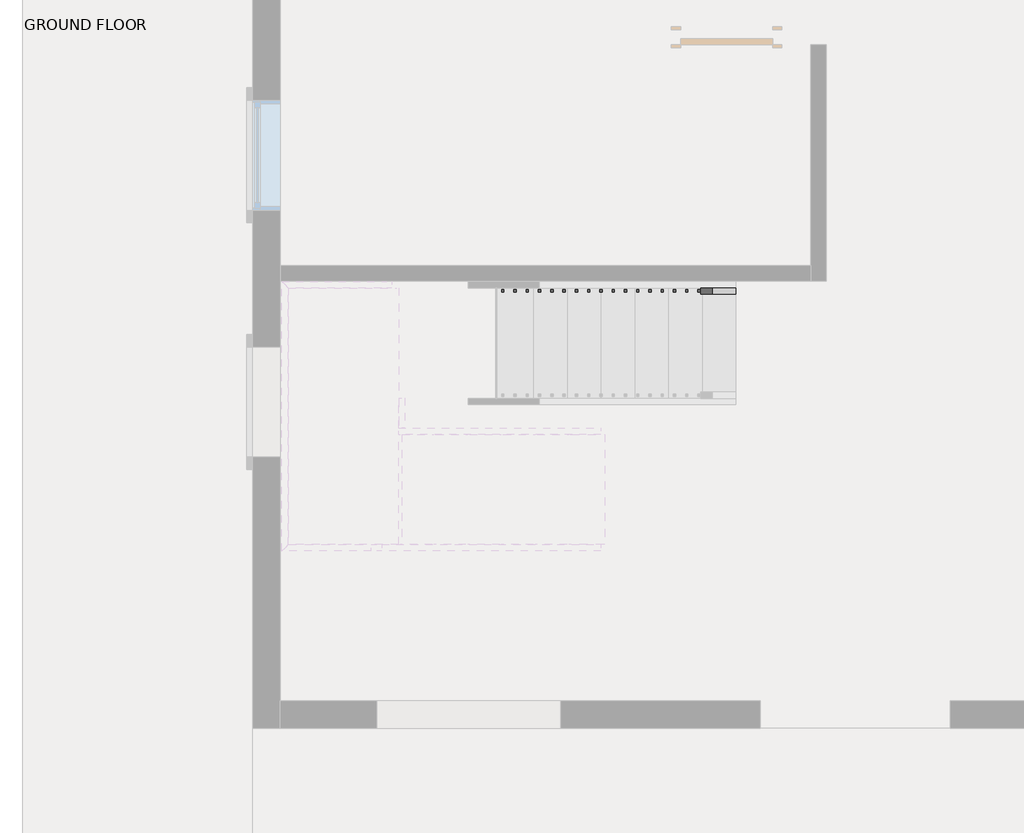
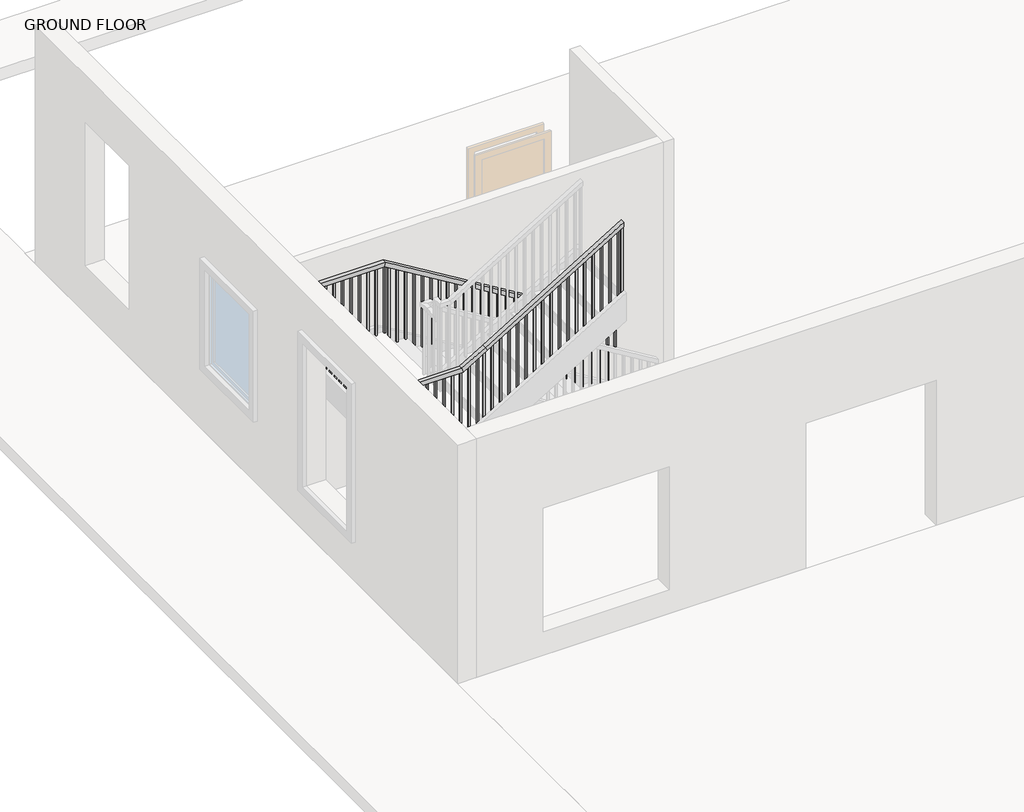
# One storey, part 2 of 3: 1 railing.
"""IFC4 building model written with IfcOpenShell, lengths in millimetres."""

from ifc_helpers import new_model, si_unit, frame, origin, place, context, project, spatial, polyline, outline, extrude, faceted_brep, element, save

model = new_model("IFC4")

# Units and contexts
model_context = context("Model", 3, world=origin())
ifc_project = project(units=[si_unit("LENGTHUNIT", "METRE", prefix="MILLI")], contexts=[model_context])

# Site, building, storey
site = spatial("IfcSite", under=ifc_project)
building = spatial("IfcBuilding", under=site)
storey = spatial("IfcBuildingStorey", under=building, Name="GROUND FLOOR", Elevation=304.8)

# Railing
placement = place(None, origin())
element("IfcRailing", 1, ObjectType="Handrail - Rectangular", at=placement, inside=storey, context=model_context, shape_type="SolidModel", body=[
    faceted_brep([(-5990.8517085, 2868.2826226, 1388.5333333), (-5990.8517085, 2868.2826226, 1329.1318731), (-5990.8517085, 2919.0826226, 1329.1318731), (-5990.8517085, 2919.0826226, 1388.5333333), (-8784.8517085, 2868.2826226, 3081.8666667), (-8799.0441179, 2868.2826226, 3031.0666667), (-8799.0441179, 2919.0826226, 3031.0666667), (-8784.8517085, 2919.0826226, 3081.8666667), (-9648.4517085, 2868.2826226, 3081.8666667), (-9648.4517085, 2868.2826226, 3031.0666667), (-9699.2517085, 2919.0826226, 3031.0666667), (-9699.2517085, 2919.0826226, 3081.8666667), (-9648.4517085, 842.8165128, 3081.8666667), (-9648.4517085, 842.8165128, 3031.0666667), (-9699.2517085, 792.0165128, 3031.0666667), (-9699.2517085, 792.0165128, 3081.8666667), (-9064.2517085, 842.8165128, 3081.8666667), (-9050.0592991, 842.8165128, 3031.0666667), (-9050.0592991, 792.0165128, 3031.0666667), (-9064.2517085, 792.0165128, 3081.8666667), (-8784.8517085, 842.8165128, 3251.2), (-8758.5219813, 842.8165128, 3207.7559502), (-8758.5219813, 792.0165128, 3207.7559502), (-8784.8517085, 792.0165128, 3251.2), (-7108.4517085, 842.8165128, 4267.2), (-7108.4517085, 792.0165128, 4267.2), (-7108.4517085, 792.0165128, 4207.7985397), (-7108.4517085, 842.8165128, 4207.7985397)], [[[0, 1, 2, 3]], [[1, 0, 4, 5]], [[2, 1, 5, 6]], [[3, 2, 6, 7]], [[0, 3, 7, 4]], [[5, 4, 8, 9]], [[6, 5, 9, 10]], [[7, 6, 10, 11]], [[4, 7, 11, 8]], [[9, 8, 12, 13]], [[10, 9, 13, 14]], [[11, 10, 14, 15]], [[8, 11, 15, 12]], [[13, 12, 16, 17]], [[14, 13, 17, 18]], [[15, 14, 18, 19]], [[12, 15, 19, 16]], [[17, 16, 20, 21]], [[18, 17, 21, 22]], [[19, 18, 22, 23]], [[16, 19, 23, 20]], [[24, 25, 26, 27]], [[21, 20, 24, 27]], [[22, 21, 27, 26]], [[23, 22, 26, 25]], [[20, 23, 25, 24]]]),
    extrude(outline(polyline([(4182.7833882, -7149.7267085), (4171.2379337, -7168.7767085), (3183.4666667, -7168.7767085), (3183.4666667, -7149.7267085), (4182.7833882, -7149.7267085)])), frame((0.0, 807.8915128, 0.0), z_axis=(0.0, 1.0, 0.0), x_axis=(0.0, 0.0, 1.0)), (0.0, 0.0, 1.0), 19.05),
    extrude(outline(polyline([(4121.2076307, -7251.3267085), (4109.6621761, -7270.3767085), (3183.4666667, -7270.3767085), (3183.4666667, -7251.3267085), (4121.2076307, -7251.3267085)])), frame((0.0, 807.8915128, 0.0), z_axis=(0.0, 1.0, 0.0), x_axis=(0.0, 0.0, 1.0)), (0.0, 0.0, 1.0), 19.05),
    extrude(outline(polyline([(4059.6318731, -7352.9267085), (4048.0864185, -7371.9767085), (3183.4666667, -7371.9767085), (3183.4666667, -7352.9267085), (4059.6318731, -7352.9267085)])), frame((0.0, 807.8915128, 0.0), z_axis=(0.0, 1.0, 0.0), x_axis=(0.0, 0.0, 1.0)), (0.0, 0.0, 1.0), 19.05),
    extrude(outline(polyline([(3998.0561155, -7454.5267085), (3986.510661, -7473.5767085), (3014.1333333, -7473.5767085), (3014.1333333, -7454.5267085), (3998.0561155, -7454.5267085)])), frame((0.0, 807.8915128, 0.0), z_axis=(0.0, 1.0, 0.0), x_axis=(0.0, 0.0, 1.0)), (0.0, 0.0, 1.0), 19.05),
    extrude(outline(polyline([(3936.4803579, -7556.1267085), (3924.9349034, -7575.1767085), (3014.1333333, -7575.1767085), (3014.1333333, -7556.1267085), (3936.4803579, -7556.1267085)])), frame((0.0, 807.8915128, 0.0), z_axis=(0.0, 1.0, 0.0), x_axis=(0.0, 0.0, 1.0)), (0.0, 0.0, 1.0), 19.05),
    extrude(outline(polyline([(3874.9046004, -7657.7267085), (3863.3591458, -7676.7767085), (3014.1333333, -7676.7767085), (3014.1333333, -7657.7267085), (3874.9046004, -7657.7267085)])), frame((0.0, 807.8915128, 0.0), z_axis=(0.0, 1.0, 0.0), x_axis=(0.0, 0.0, 1.0)), (0.0, 0.0, 1.0), 19.05),
    extrude(outline(polyline([(3813.3288428, -7759.3267085), (3801.7833882, -7778.3767085), (2844.8, -7778.3767085), (2844.8, -7759.3267085), (3813.3288428, -7759.3267085)])), frame((0.0, 807.8915128, 0.0), z_axis=(0.0, 1.0, 0.0), x_axis=(0.0, 0.0, 1.0)), (0.0, 0.0, 1.0), 19.05),
    extrude(outline(polyline([(3751.7530852, -7860.9267085), (3740.2076307, -7879.9767085), (2844.8, -7879.9767085), (2844.8, -7860.9267085), (3751.7530852, -7860.9267085)])), frame((0.0, 807.8915128, 0.0), z_axis=(0.0, 1.0, 0.0), x_axis=(0.0, 0.0, 1.0)), (0.0, 0.0, 1.0), 19.05),
    extrude(outline(polyline([(3690.1773276, -7962.5267085), (3678.6318731, -7981.5767085), (2675.4666667, -7981.5767085), (2675.4666667, -7962.5267085), (3690.1773276, -7962.5267085)])), frame((0.0, 807.8915128, 0.0), z_axis=(0.0, 1.0, 0.0), x_axis=(0.0, 0.0, 1.0)), (0.0, 0.0, 1.0), 19.05),
    extrude(outline(polyline([(3628.60157, -8064.1267085), (3617.0561155, -8083.1767085), (2675.4666667, -8083.1767085), (2675.4666667, -8064.1267085), (3628.60157, -8064.1267085)])), frame((0.0, 807.8915128, 0.0), z_axis=(0.0, 1.0, 0.0), x_axis=(0.0, 0.0, 1.0)), (0.0, 0.0, 1.0), 19.05),
    extrude(outline(polyline([(3567.0258125, -8165.7267085), (3555.4803579, -8184.7767085), (2675.4666667, -8184.7767085), (2675.4666667, -8165.7267085), (3567.0258125, -8165.7267085)])), frame((0.0, 807.8915128, 0.0), z_axis=(0.0, 1.0, 0.0), x_axis=(0.0, 0.0, 1.0)), (0.0, 0.0, 1.0), 19.05),
    extrude(outline(polyline([(3505.4500549, -8267.3267085), (3493.9046004, -8286.3767085), (2506.1333333, -8286.3767085), (2506.1333333, -8267.3267085), (3505.4500549, -8267.3267085)])), frame((0.0, 807.8915128, 0.0), z_axis=(0.0, 1.0, 0.0), x_axis=(0.0, 0.0, 1.0)), (0.0, 0.0, 1.0), 19.05),
    extrude(outline(polyline([(3443.8742973, -8368.9267085), (3432.3288428, -8387.9767085), (2506.1333333, -8387.9767085), (2506.1333333, -8368.9267085), (3443.8742973, -8368.9267085)])), frame((0.0, 807.8915128, 0.0), z_axis=(0.0, 1.0, 0.0), x_axis=(0.0, 0.0, 1.0)), (0.0, 0.0, 1.0), 19.05),
    extrude(outline(polyline([(3382.2985397, -8470.5267085), (3370.7530852, -8489.5767085), (2506.1333333, -8489.5767085), (2506.1333333, -8470.5267085), (3382.2985397, -8470.5267085)])), frame((0.0, 807.8915128, 0.0), z_axis=(0.0, 1.0, 0.0), x_axis=(0.0, 0.0, 1.0)), (0.0, 0.0, 1.0), 19.05),
    extrude(outline(polyline([(3320.7227822, -8572.1267085), (3309.1773276, -8591.1767085), (2336.8, -8591.1767085), (2336.8, -8572.1267085), (3320.7227822, -8572.1267085)])), frame((0.0, 807.8915128, 0.0), z_axis=(0.0, 1.0, 0.0), x_axis=(0.0, 0.0, 1.0)), (0.0, 0.0, 1.0), 19.05),
    extrude(outline(polyline([(3259.1470246, -8673.7267085), (3247.60157, -8692.7767085), (2336.8, -8692.7767085), (2336.8, -8673.7267085), (3259.1470246, -8673.7267085)])), frame((0.0, 807.8915128, 0.0), z_axis=(0.0, 1.0, 0.0), x_axis=(0.0, 0.0, 1.0)), (0.0, 0.0, 1.0), 19.05),
    extrude(outline(polyline([(3151.3894488, -8851.5267085), (3139.8439943, -8870.5767085), (2167.4666667, -8870.5767085), (2167.4666667, -8851.5267085), (3151.3894488, -8851.5267085)])), frame((0.0, 807.8915128, 0.0), z_axis=(0.0, 1.0, 0.0), x_axis=(0.0, 0.0, 1.0)), (0.0, 0.0, 1.0), 19.05),
    extrude(outline(polyline([(3089.8136913, -8953.1267085), (3078.2682367, -8972.1767085), (2167.4666667, -8972.1767085), (2167.4666667, -8953.1267085), (3089.8136913, -8953.1267085)])), frame((0.0, 807.8915128, 0.0), z_axis=(0.0, 1.0, 0.0), x_axis=(0.0, 0.0, 1.0)), (0.0, 0.0, 1.0), 19.05),
    extrude(outline(polyline([(-9073.7767085, 807.8915128), (-9073.7767085, 826.9415128), (-9054.7267085, 826.9415128), (-9054.7267085, 807.8915128), (-9073.7767085, 807.8915128)])), frame((0.0, 0.0, 2167.4666667), z_axis=(0.0, 0.0, 1.0), x_axis=(1.0, 0.0, 0.0)), (0.0, 0.0, 1.0), 863.6),
    extrude(outline(polyline([(-9175.3767085, 807.8915128), (-9175.3767085, 826.9415128), (-9156.3267085, 826.9415128), (-9156.3267085, 807.8915128), (-9175.3767085, 807.8915128)])), frame((0.0, 0.0, 2167.4666667), z_axis=(0.0, 0.0, 1.0), x_axis=(1.0, 0.0, 0.0)), (0.0, 0.0, 1.0), 863.6),
    extrude(outline(polyline([(-9276.9767085, 807.8915128), (-9276.9767085, 826.9415128), (-9257.9267085, 826.9415128), (-9257.9267085, 807.8915128), (-9276.9767085, 807.8915128)])), frame((0.0, 0.0, 2167.4666667), z_axis=(0.0, 0.0, 1.0), x_axis=(1.0, 0.0, 0.0)), (0.0, 0.0, 1.0), 863.6),
    extrude(outline(polyline([(-9378.5767085, 807.8915128), (-9378.5767085, 826.9415128), (-9359.5267085, 826.9415128), (-9359.5267085, 807.8915128), (-9378.5767085, 807.8915128)])), frame((0.0, 0.0, 2167.4666667), z_axis=(0.0, 0.0, 1.0), x_axis=(1.0, 0.0, 0.0)), (0.0, 0.0, 1.0), 863.6),
    extrude(outline(polyline([(-9480.1767085, 807.8915128), (-9480.1767085, 826.9415128), (-9461.1267085, 826.9415128), (-9461.1267085, 807.8915128), (-9480.1767085, 807.8915128)])), frame((0.0, 0.0, 2167.4666667), z_axis=(0.0, 0.0, 1.0), x_axis=(1.0, 0.0, 0.0)), (0.0, 0.0, 1.0), 863.6),
    extrude(outline(polyline([(-9581.7767085, 807.8915128), (-9581.7767085, 826.9415128), (-9562.7267085, 826.9415128), (-9562.7267085, 807.8915128), (-9581.7767085, 807.8915128)])), frame((0.0, 0.0, 2167.4666667), z_axis=(0.0, 0.0, 1.0), x_axis=(1.0, 0.0, 0.0)), (0.0, 0.0, 1.0), 863.6),
    extrude(outline(polyline([(-9683.3767085, 871.2076226), (-9664.3267085, 871.2076226), (-9664.3267085, 852.1576226), (-9683.3767085, 852.1576226), (-9683.3767085, 871.2076226)])), frame((0.0, 0.0, 2167.4666667), z_axis=(0.0, 0.0, 1.0), x_axis=(1.0, 0.0, 0.0)), (0.0, 0.0, 1.0), 863.6),
    extrude(outline(polyline([(-9683.3767085, 972.8076226), (-9664.3267085, 972.8076226), (-9664.3267085, 953.7576226), (-9683.3767085, 953.7576226), (-9683.3767085, 972.8076226)])), frame((0.0, 0.0, 2167.4666667), z_axis=(0.0, 0.0, 1.0), x_axis=(1.0, 0.0, 0.0)), (0.0, 0.0, 1.0), 863.6),
    extrude(outline(polyline([(-9683.3767085, 1074.4076226), (-9664.3267085, 1074.4076226), (-9664.3267085, 1055.3576226), (-9683.3767085, 1055.3576226), (-9683.3767085, 1074.4076226)])), frame((0.0, 0.0, 2167.4666667), z_axis=(0.0, 0.0, 1.0), x_axis=(1.0, 0.0, 0.0)), (0.0, 0.0, 1.0), 863.6),
    extrude(outline(polyline([(-9683.3767085, 1176.0076226), (-9664.3267085, 1176.0076226), (-9664.3267085, 1156.9576226), (-9683.3767085, 1156.9576226), (-9683.3767085, 1176.0076226)])), frame((0.0, 0.0, 2167.4666667), z_axis=(0.0, 0.0, 1.0), x_axis=(1.0, 0.0, 0.0)), (0.0, 0.0, 1.0), 863.6),
    extrude(outline(polyline([(-9683.3767085, 1277.6076226), (-9664.3267085, 1277.6076226), (-9664.3267085, 1258.5576226), (-9683.3767085, 1258.5576226), (-9683.3767085, 1277.6076226)])), frame((0.0, 0.0, 2167.4666667), z_axis=(0.0, 0.0, 1.0), x_axis=(1.0, 0.0, 0.0)), (0.0, 0.0, 1.0), 863.6),
    extrude(outline(polyline([(-9683.3767085, 1379.2076226), (-9664.3267085, 1379.2076226), (-9664.3267085, 1360.1576226), (-9683.3767085, 1360.1576226), (-9683.3767085, 1379.2076226)])), frame((0.0, 0.0, 2167.4666667), z_axis=(0.0, 0.0, 1.0), x_axis=(1.0, 0.0, 0.0)), (0.0, 0.0, 1.0), 863.6),
    extrude(outline(polyline([(-9683.3767085, 1480.8076226), (-9664.3267085, 1480.8076226), (-9664.3267085, 1461.7576226), (-9683.3767085, 1461.7576226), (-9683.3767085, 1480.8076226)])), frame((0.0, 0.0, 2167.4666667), z_axis=(0.0, 0.0, 1.0), x_axis=(1.0, 0.0, 0.0)), (0.0, 0.0, 1.0), 863.6),
    extrude(outline(polyline([(-9683.3767085, 1582.4076226), (-9664.3267085, 1582.4076226), (-9664.3267085, 1563.3576226), (-9683.3767085, 1563.3576226), (-9683.3767085, 1582.4076226)])), frame((0.0, 0.0, 2167.4666667), z_axis=(0.0, 0.0, 1.0), x_axis=(1.0, 0.0, 0.0)), (0.0, 0.0, 1.0), 863.6),
    extrude(outline(polyline([(-9683.3767085, 1684.0076226), (-9664.3267085, 1684.0076226), (-9664.3267085, 1664.9576226), (-9683.3767085, 1664.9576226), (-9683.3767085, 1684.0076226)])), frame((0.0, 0.0, 2167.4666667), z_axis=(0.0, 0.0, 1.0), x_axis=(1.0, 0.0, 0.0)), (0.0, 0.0, 1.0), 863.6),
    extrude(outline(polyline([(-9683.3767085, 1785.6076226), (-9664.3267085, 1785.6076226), (-9664.3267085, 1766.5576226), (-9683.3767085, 1766.5576226), (-9683.3767085, 1785.6076226)])), frame((0.0, 0.0, 2167.4666667), z_axis=(0.0, 0.0, 1.0), x_axis=(1.0, 0.0, 0.0)), (0.0, 0.0, 1.0), 863.6),
    extrude(outline(polyline([(-9683.3767085, 1887.2076226), (-9664.3267085, 1887.2076226), (-9664.3267085, 1868.1576226), (-9683.3767085, 1868.1576226), (-9683.3767085, 1887.2076226)])), frame((0.0, 0.0, 2167.4666667), z_axis=(0.0, 0.0, 1.0), x_axis=(1.0, 0.0, 0.0)), (0.0, 0.0, 1.0), 863.6),
    extrude(outline(polyline([(-9683.3767085, 1988.8076226), (-9664.3267085, 1988.8076226), (-9664.3267085, 1969.7576226), (-9683.3767085, 1969.7576226), (-9683.3767085, 1988.8076226)])), frame((0.0, 0.0, 2167.4666667), z_axis=(0.0, 0.0, 1.0), x_axis=(1.0, 0.0, 0.0)), (0.0, 0.0, 1.0), 863.6),
    extrude(outline(polyline([(-9683.3767085, 2090.4076226), (-9664.3267085, 2090.4076226), (-9664.3267085, 2071.3576226), (-9683.3767085, 2071.3576226), (-9683.3767085, 2090.4076226)])), frame((0.0, 0.0, 2167.4666667), z_axis=(0.0, 0.0, 1.0), x_axis=(1.0, 0.0, 0.0)), (0.0, 0.0, 1.0), 863.6),
    extrude(outline(polyline([(-9683.3767085, 2192.0076226), (-9664.3267085, 2192.0076226), (-9664.3267085, 2172.9576226), (-9683.3767085, 2172.9576226), (-9683.3767085, 2192.0076226)])), frame((0.0, 0.0, 2167.4666667), z_axis=(0.0, 0.0, 1.0), x_axis=(1.0, 0.0, 0.0)), (0.0, 0.0, 1.0), 863.6),
    extrude(outline(polyline([(-9683.3767085, 2293.6076226), (-9664.3267085, 2293.6076226), (-9664.3267085, 2274.5576226), (-9683.3767085, 2274.5576226), (-9683.3767085, 2293.6076226)])), frame((0.0, 0.0, 2167.4666667), z_axis=(0.0, 0.0, 1.0), x_axis=(1.0, 0.0, 0.0)), (0.0, 0.0, 1.0), 863.6),
    extrude(outline(polyline([(-9683.3767085, 2395.2076226), (-9664.3267085, 2395.2076226), (-9664.3267085, 2376.1576226), (-9683.3767085, 2376.1576226), (-9683.3767085, 2395.2076226)])), frame((0.0, 0.0, 2167.4666667), z_axis=(0.0, 0.0, 1.0), x_axis=(1.0, 0.0, 0.0)), (0.0, 0.0, 1.0), 863.6),
    extrude(outline(polyline([(-9683.3767085, 2496.8076226), (-9664.3267085, 2496.8076226), (-9664.3267085, 2477.7576226), (-9683.3767085, 2477.7576226), (-9683.3767085, 2496.8076226)])), frame((0.0, 0.0, 2167.4666667), z_axis=(0.0, 0.0, 1.0), x_axis=(1.0, 0.0, 0.0)), (0.0, 0.0, 1.0), 863.6),
    extrude(outline(polyline([(-9683.3767085, 2598.4076226), (-9664.3267085, 2598.4076226), (-9664.3267085, 2579.3576226), (-9683.3767085, 2579.3576226), (-9683.3767085, 2598.4076226)])), frame((0.0, 0.0, 2167.4666667), z_axis=(0.0, 0.0, 1.0), x_axis=(1.0, 0.0, 0.0)), (0.0, 0.0, 1.0), 863.6),
    extrude(outline(polyline([(-9683.3767085, 2700.0076226), (-9664.3267085, 2700.0076226), (-9664.3267085, 2680.9576226), (-9683.3767085, 2680.9576226), (-9683.3767085, 2700.0076226)])), frame((0.0, 0.0, 2167.4666667), z_axis=(0.0, 0.0, 1.0), x_axis=(1.0, 0.0, 0.0)), (0.0, 0.0, 1.0), 863.6),
    extrude(outline(polyline([(-9683.3767085, 2801.6076226), (-9664.3267085, 2801.6076226), (-9664.3267085, 2782.5576226), (-9683.3767085, 2782.5576226), (-9683.3767085, 2801.6076226)])), frame((0.0, 0.0, 2167.4666667), z_axis=(0.0, 0.0, 1.0), x_axis=(1.0, 0.0, 0.0)), (0.0, 0.0, 1.0), 863.6),
    extrude(outline(polyline([(-9588.1267085, 2903.2076226), (-9588.1267085, 2884.1576226), (-9607.1767085, 2884.1576226), (-9607.1767085, 2903.2076226), (-9588.1267085, 2903.2076226)])), frame((0.0, 0.0, 2167.4666667), z_axis=(0.0, 0.0, 1.0), x_axis=(1.0, 0.0, 0.0)), (0.0, 0.0, 1.0), 863.6),
    extrude(outline(polyline([(-9486.5267085, 2903.2076226), (-9486.5267085, 2884.1576226), (-9505.5767085, 2884.1576226), (-9505.5767085, 2903.2076226), (-9486.5267085, 2903.2076226)])), frame((0.0, 0.0, 2167.4666667), z_axis=(0.0, 0.0, 1.0), x_axis=(1.0, 0.0, 0.0)), (0.0, 0.0, 1.0), 863.6),
    extrude(outline(polyline([(-9384.9267085, 2903.2076226), (-9384.9267085, 2884.1576226), (-9403.9767085, 2884.1576226), (-9403.9767085, 2903.2076226), (-9384.9267085, 2903.2076226)])), frame((0.0, 0.0, 2167.4666667), z_axis=(0.0, 0.0, 1.0), x_axis=(1.0, 0.0, 0.0)), (0.0, 0.0, 1.0), 863.6),
    extrude(outline(polyline([(-9283.3267085, 2903.2076226), (-9283.3267085, 2884.1576226), (-9302.3767085, 2884.1576226), (-9302.3767085, 2903.2076226), (-9283.3267085, 2903.2076226)])), frame((0.0, 0.0, 2167.4666667), z_axis=(0.0, 0.0, 1.0), x_axis=(1.0, 0.0, 0.0)), (0.0, 0.0, 1.0), 863.6),
    extrude(outline(polyline([(-9181.7267085, 2903.2076226), (-9181.7267085, 2884.1576226), (-9200.7767085, 2884.1576226), (-9200.7767085, 2903.2076226), (-9181.7267085, 2903.2076226)])), frame((0.0, 0.0, 2167.4666667), z_axis=(0.0, 0.0, 1.0), x_axis=(1.0, 0.0, 0.0)), (0.0, 0.0, 1.0), 863.6),
    extrude(outline(polyline([(-9080.1267085, 2903.2076226), (-9080.1267085, 2884.1576226), (-9099.1767085, 2884.1576226), (-9099.1767085, 2903.2076226), (-9080.1267085, 2903.2076226)])), frame((0.0, 0.0, 2167.4666667), z_axis=(0.0, 0.0, 1.0), x_axis=(1.0, 0.0, 0.0)), (0.0, 0.0, 1.0), 863.6),
    extrude(outline(polyline([(-8978.5267085, 2903.2076226), (-8978.5267085, 2884.1576226), (-8997.5767085, 2884.1576226), (-8997.5767085, 2903.2076226), (-8978.5267085, 2903.2076226)])), frame((0.0, 0.0, 2167.4666667), z_axis=(0.0, 0.0, 1.0), x_axis=(1.0, 0.0, 0.0)), (0.0, 0.0, 1.0), 863.6),
    extrude(outline(polyline([(-8876.9267085, 2903.2076226), (-8876.9267085, 2884.1576226), (-8895.9767085, 2884.1576226), (-8895.9767085, 2903.2076226), (-8876.9267085, 2903.2076226)])), frame((0.0, 0.0, 2167.4666667), z_axis=(0.0, 0.0, 1.0), x_axis=(1.0, 0.0, 0.0)), (0.0, 0.0, 1.0), 863.6),
    extrude(outline(polyline([(2985.9046004, -8724.5267085), (2997.4500549, -8743.5767085), (1998.1333333, -8743.5767085), (1998.1333333, -8724.5267085), (2985.9046004, -8724.5267085)])), frame((0.0, 2884.1576226, 0.0), z_axis=(0.0, 1.0, 0.0), x_axis=(0.0, 0.0, 1.0)), (0.0, 0.0, 1.0), 19.05),
    extrude(outline(polyline([(2924.3288428, -8622.9267085), (2935.8742973, -8641.9767085), (1998.1333333, -8641.9767085), (1998.1333333, -8622.9267085), (2924.3288428, -8622.9267085)])), frame((0.0, 2884.1576226, 0.0), z_axis=(0.0, 1.0, 0.0), x_axis=(0.0, 0.0, 1.0)), (0.0, 0.0, 1.0), 19.05),
    extrude(outline(polyline([(2862.7530852, -8521.3267085), (2874.2985397, -8540.3767085), (1998.1333333, -8540.3767085), (1998.1333333, -8521.3267085), (2862.7530852, -8521.3267085)])), frame((0.0, 2884.1576226, 0.0), z_axis=(0.0, 1.0, 0.0), x_axis=(0.0, 0.0, 1.0)), (0.0, 0.0, 1.0), 19.05),
    extrude(outline(polyline([(2801.1773276, -8419.7267085), (2812.7227822, -8438.7767085), (1828.8, -8438.7767085), (1828.8, -8419.7267085), (2801.1773276, -8419.7267085)])), frame((0.0, 2884.1576226, 0.0), z_axis=(0.0, 1.0, 0.0), x_axis=(0.0, 0.0, 1.0)), (0.0, 0.0, 1.0), 19.05),
    extrude(outline(polyline([(2739.60157, -8318.1267085), (2751.1470246, -8337.1767085), (1828.8, -8337.1767085), (1828.8, -8318.1267085), (2739.60157, -8318.1267085)])), frame((0.0, 2884.1576226, 0.0), z_axis=(0.0, 1.0, 0.0), x_axis=(0.0, 0.0, 1.0)), (0.0, 0.0, 1.0), 19.05),
    extrude(outline(polyline([(2678.0258125, -8216.5267085), (2689.571267, -8235.5767085), (1828.8, -8235.5767085), (1828.8, -8216.5267085), (2678.0258125, -8216.5267085)])), frame((0.0, 2884.1576226, 0.0), z_axis=(0.0, 1.0, 0.0), x_axis=(0.0, 0.0, 1.0)), (0.0, 0.0, 1.0), 19.05),
    extrude(outline(polyline([(2616.4500549, -8114.9267085), (2627.9955094, -8133.9767085), (1659.4666667, -8133.9767085), (1659.4666667, -8114.9267085), (2616.4500549, -8114.9267085)])), frame((0.0, 2884.1576226, 0.0), z_axis=(0.0, 1.0, 0.0), x_axis=(0.0, 0.0, 1.0)), (0.0, 0.0, 1.0), 19.05),
    extrude(outline(polyline([(2554.8742973, -8013.3267085), (2566.4197519, -8032.3767085), (1659.4666667, -8032.3767085), (1659.4666667, -8013.3267085), (2554.8742973, -8013.3267085)])), frame((0.0, 2884.1576226, 0.0), z_axis=(0.0, 1.0, 0.0), x_axis=(0.0, 0.0, 1.0)), (0.0, 0.0, 1.0), 19.05),
    extrude(outline(polyline([(2493.2985397, -7911.7267085), (2504.8439943, -7930.7767085), (1490.1333333, -7930.7767085), (1490.1333333, -7911.7267085), (2493.2985397, -7911.7267085)])), frame((0.0, 2884.1576226, 0.0), z_axis=(0.0, 1.0, 0.0), x_axis=(0.0, 0.0, 1.0)), (0.0, 0.0, 1.0), 19.05),
    extrude(outline(polyline([(2431.7227822, -7810.1267085), (2443.2682367, -7829.1767085), (1490.1333333, -7829.1767085), (1490.1333333, -7810.1267085), (2431.7227822, -7810.1267085)])), frame((0.0, 2884.1576226, 0.0), z_axis=(0.0, 1.0, 0.0), x_axis=(0.0, 0.0, 1.0)), (0.0, 0.0, 1.0), 19.05),
    extrude(outline(polyline([(2370.1470246, -7708.5267085), (2381.6924791, -7727.5767085), (1490.1333333, -7727.5767085), (1490.1333333, -7708.5267085), (2370.1470246, -7708.5267085)])), frame((0.0, 2884.1576226, 0.0), z_axis=(0.0, 1.0, 0.0), x_axis=(0.0, 0.0, 1.0)), (0.0, 0.0, 1.0), 19.05),
    extrude(outline(polyline([(2308.571267, -7606.9267085), (2320.1167216, -7625.9767085), (1320.8, -7625.9767085), (1320.8, -7606.9267085), (2308.571267, -7606.9267085)])), frame((0.0, 2884.1576226, 0.0), z_axis=(0.0, 1.0, 0.0), x_axis=(0.0, 0.0, 1.0)), (0.0, 0.0, 1.0), 19.05),
    extrude(outline(polyline([(2246.9955094, -7505.3267085), (2258.540964, -7524.3767085), (1320.8, -7524.3767085), (1320.8, -7505.3267085), (2246.9955094, -7505.3267085)])), frame((0.0, 2884.1576226, 0.0), z_axis=(0.0, 1.0, 0.0), x_axis=(0.0, 0.0, 1.0)), (0.0, 0.0, 1.0), 19.05),
    extrude(outline(polyline([(2185.4197519, -7403.7267085), (2196.9652064, -7422.7767085), (1320.8, -7422.7767085), (1320.8, -7403.7267085), (2185.4197519, -7403.7267085)])), frame((0.0, 2884.1576226, 0.0), z_axis=(0.0, 1.0, 0.0), x_axis=(0.0, 0.0, 1.0)), (0.0, 0.0, 1.0), 19.05),
    extrude(outline(polyline([(2123.8439943, -7302.1267085), (2135.3894488, -7321.1767085), (1151.4666667, -7321.1767085), (1151.4666667, -7302.1267085), (2123.8439943, -7302.1267085)])), frame((0.0, 2884.1576226, 0.0), z_axis=(0.0, 1.0, 0.0), x_axis=(0.0, 0.0, 1.0)), (0.0, 0.0, 1.0), 19.05),
    extrude(outline(polyline([(2062.2682367, -7200.5267085), (2073.8136913, -7219.5767085), (1151.4666667, -7219.5767085), (1151.4666667, -7200.5267085), (2062.2682367, -7200.5267085)])), frame((0.0, 2884.1576226, 0.0), z_axis=(0.0, 1.0, 0.0), x_axis=(0.0, 0.0, 1.0)), (0.0, 0.0, 1.0), 19.05),
    extrude(outline(polyline([(2000.6924791, -7098.9267085), (2012.2379337, -7117.9767085), (1151.4666667, -7117.9767085), (1151.4666667, -7098.9267085), (2000.6924791, -7098.9267085)])), frame((0.0, 2884.1576226, 0.0), z_axis=(0.0, 1.0, 0.0), x_axis=(0.0, 0.0, 1.0)), (0.0, 0.0, 1.0), 19.05),
    extrude(outline(polyline([(1939.1167216, -6997.3267085), (1950.6621761, -7016.3767085), (982.1333333, -7016.3767085), (982.1333333, -6997.3267085), (1939.1167216, -6997.3267085)])), frame((0.0, 2884.1576226, 0.0), z_axis=(0.0, 1.0, 0.0), x_axis=(0.0, 0.0, 1.0)), (0.0, 0.0, 1.0), 19.05),
    extrude(outline(polyline([(1877.540964, -6895.7267085), (1889.0864185, -6914.7767085), (982.1333333, -6914.7767085), (982.1333333, -6895.7267085), (1877.540964, -6895.7267085)])), frame((0.0, 2884.1576226, 0.0), z_axis=(0.0, 1.0, 0.0), x_axis=(0.0, 0.0, 1.0)), (0.0, 0.0, 1.0), 19.05),
    extrude(outline(polyline([(1815.9652064, -6794.1267085), (1827.510661, -6813.1767085), (812.8, -6813.1767085), (812.8, -6794.1267085), (1815.9652064, -6794.1267085)])), frame((0.0, 2884.1576226, 0.0), z_axis=(0.0, 1.0, 0.0), x_axis=(0.0, 0.0, 1.0)), (0.0, 0.0, 1.0), 19.05),
    extrude(outline(polyline([(1754.3894488, -6692.5267085), (1765.9349034, -6711.5767085), (812.8, -6711.5767085), (812.8, -6692.5267085), (1754.3894488, -6692.5267085)])), frame((0.0, 2884.1576226, 0.0), z_axis=(0.0, 1.0, 0.0), x_axis=(0.0, 0.0, 1.0)), (0.0, 0.0, 1.0), 19.05),
    extrude(outline(polyline([(1692.8136913, -6590.9267085), (1704.3591458, -6609.9767085), (812.8, -6609.9767085), (812.8, -6590.9267085), (1692.8136913, -6590.9267085)])), frame((0.0, 2884.1576226, 0.0), z_axis=(0.0, 1.0, 0.0), x_axis=(0.0, 0.0, 1.0)), (0.0, 0.0, 1.0), 19.05),
    extrude(outline(polyline([(1631.2379337, -6489.3267085), (1642.7833882, -6508.3767085), (643.4666667, -6508.3767085), (643.4666667, -6489.3267085), (1631.2379337, -6489.3267085)])), frame((0.0, 2884.1576226, 0.0), z_axis=(0.0, 1.0, 0.0), x_axis=(0.0, 0.0, 1.0)), (0.0, 0.0, 1.0), 19.05),
    extrude(outline(polyline([(1569.6621761, -6387.7267085), (1581.2076307, -6406.7767085), (643.4666667, -6406.7767085), (643.4666667, -6387.7267085), (1569.6621761, -6387.7267085)])), frame((0.0, 2884.1576226, 0.0), z_axis=(0.0, 1.0, 0.0), x_axis=(0.0, 0.0, 1.0)), (0.0, 0.0, 1.0), 19.05),
    extrude(outline(polyline([(1508.0864185, -6286.1267085), (1519.6318731, -6305.1767085), (643.4666667, -6305.1767085), (643.4666667, -6286.1267085), (1508.0864185, -6286.1267085)])), frame((0.0, 2884.1576226, 0.0), z_axis=(0.0, 1.0, 0.0), x_axis=(0.0, 0.0, 1.0)), (0.0, 0.0, 1.0), 19.05),
    extrude(outline(polyline([(1446.510661, -6184.5267085), (1458.0561155, -6203.5767085), (474.1333333, -6203.5767085), (474.1333333, -6184.5267085), (1446.510661, -6184.5267085)])), frame((0.0, 2884.1576226, 0.0), z_axis=(0.0, 1.0, 0.0), x_axis=(0.0, 0.0, 1.0)), (0.0, 0.0, 1.0), 19.05),
    extrude(outline(polyline([(1384.9349034, -6082.9267085), (1396.4803579, -6101.9767085), (474.1333333, -6101.9767085), (474.1333333, -6082.9267085), (1384.9349034, -6082.9267085)])), frame((0.0, 2884.1576226, 0.0), z_axis=(0.0, 1.0, 0.0), x_axis=(0.0, 0.0, 1.0)), (0.0, 0.0, 1.0), 19.05),
    extrude(outline(polyline([(3197.571267, -8775.3267085), (3186.0258125, -8794.3767085), (2167.4666667, -8794.3767085), (2167.4666667, -8775.3267085), (3197.571267, -8775.3267085)])), frame((0.0, 807.8915128, 0.0), z_axis=(0.0, 1.0, 0.0), x_axis=(0.0, 0.0, 1.0)), (0.0, 0.0, 1.0), 19.05),
    extrude(outline(polyline([(-9683.3767085, 826.9415128), (-9664.3267085, 826.9415128), (-9664.3267085, 807.8915128), (-9683.3767085, 807.8915128), (-9683.3767085, 826.9415128)])), frame((0.0, 0.0, 2167.4666667), z_axis=(0.0, 0.0, 1.0), x_axis=(1.0, 0.0, 0.0)), (0.0, 0.0, 1.0), 863.6),
    extrude(outline(polyline([(-9664.3267085, 2903.2076226), (-9664.3267085, 2884.1576226), (-9683.3767085, 2884.1576226), (-9683.3767085, 2903.2076226), (-9664.3267085, 2903.2076226)])), frame((0.0, 0.0, 2167.4666667), z_axis=(0.0, 0.0, 1.0), x_axis=(1.0, 0.0, 0.0)), (0.0, 0.0, 1.0), 863.6),
    extrude(outline(polyline([(3016.6924791, -8775.3267085), (3028.2379337, -8794.3767085), (2167.4666667, -8794.3767085), (2167.4666667, -8775.3267085), (3016.6924791, -8775.3267085)])), frame((0.0, 2884.1576226, 0.0), z_axis=(0.0, 1.0, 0.0), x_axis=(0.0, 0.0, 1.0)), (0.0, 0.0, 1.0), 19.05),
    extrude(outline(polyline([(4207.7985397, -7108.4517085), (4196.2530852, -7127.5017085), (3183.4666667, -7127.5017085), (3183.4666667, -7108.4517085), (4207.7985397, -7108.4517085)])), frame((0.0, 807.8915128, 0.0), z_axis=(0.0, 1.0, 0.0), x_axis=(0.0, 0.0, 1.0)), (0.0, 0.0, 1.0), 19.05),
    extrude(outline(polyline([(1329.1318731, -5990.8517085), (1340.6773276, -6009.9017085), (474.1333333, -6009.9017085), (474.1333333, -5990.8517085), (1329.1318731, -5990.8517085)])), frame((0.0, 2884.1576226, 0.0), z_axis=(0.0, 1.0, 0.0), x_axis=(0.0, 0.0, 1.0)), (0.0, 0.0, 1.0), 19.05),
])

save(model, "model.ifc")

# Revit data of these elements
# Type "Handrail - Rectangular"
#   Assembly Code = "C2010400"
#   built-in parameter 1008612 = 0.0416667 (stored number, unit not read)
#   built-in parameter 1008611 = 0.0416667 (stored number, unit not read)
#   built-in parameter 1008609 = 0.333333 (stored number, unit not read)
#   built-in parameter 1008604 = 0.166667 (stored number, unit not read)
#   built-in parameter 1008603 = 0.166667 (stored number, unit not read)
#   Railing Height = 3' - 0"
#   built-in parameter 1008630 = 2
#   built-in parameter 1008610 = 2
#   built-in parameter 1008618 = Baluster - Square : 3/4"
# Element 1 (IfcRailing, "Handrail - Rectangular")
#   Phase Created = New Construction
